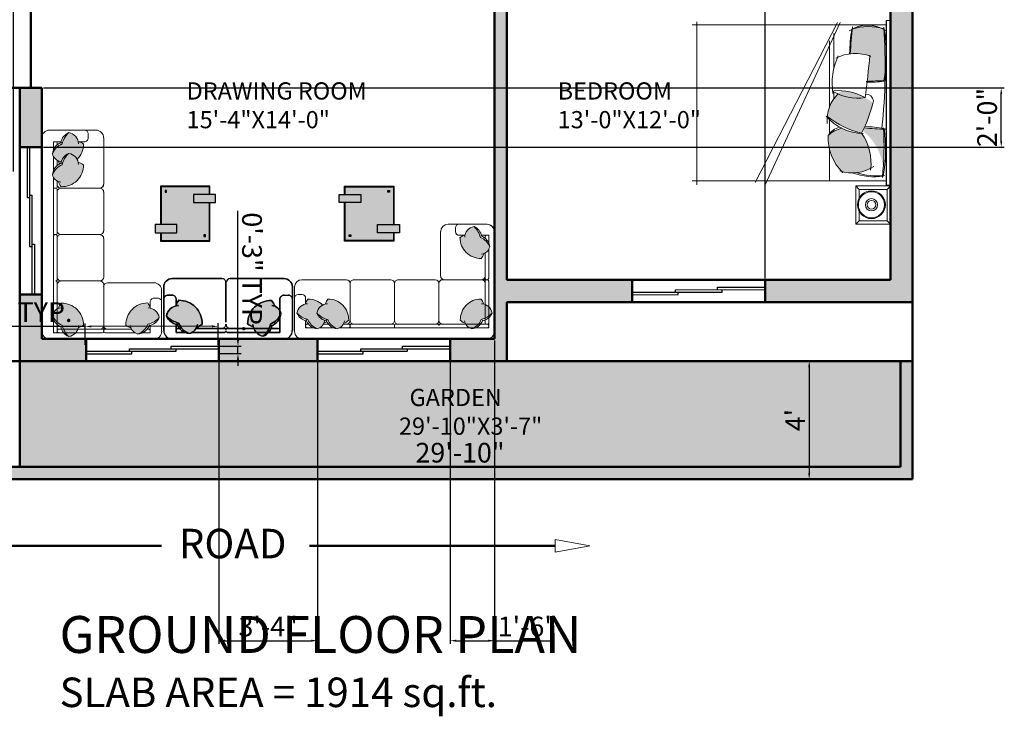
# Model space of a CAD drawing. Units: inches. Extents: x 1913 to 5309, y 1003 to 1733.
# Tile 14 of 23: x 4152 to 4552, y 1003 to 1286. Entities that reach past the tile are written whole.
import ezdxf

# ---------------------------------------------------------------- set-up
doc = ezdxf.new("R2010")
doc.units = ezdxf.units.IN
for name, color, linetype, lineweight in [('0.10', 252, 'Continuous', 9), ('0.15', 34, 'Continuous', 15), ('A-ANNO-DIMS', 2, 'Continuous', 18), ('A-ANNO-SYMB', 1, 'Continuous', 18), ('A-ANNO-TEXT', 7, 'Continuous', 18), ('A-AREA-IDEN', 3, 'Continuous', 18), ('A-DOOR', 4, 'Continuous', 25), ('A-FLOR-PATT', 252, 'Continuous', 13), ('A-FURN', 8, 'Continuous', 18), ('A-FURN-PATT', 8, 'Continuous', 13), ('A-GLAZ', 5, 'Continuous', 25), ('A-WALL', 7, 'Continuous', 50)]:
    doc.layers.add(name, color=color, linetype=linetype, lineweight=lineweight)
doc.layers.add('MOBIL', color=7, linetype='Continuous')
doc.styles.get("Standard").update_dxf_attribs({"font": 'arial.ttf'})
doc.dimstyles.new('ISO-25', dxfattribs={"dimtxt": 8, "dimasz": 2.5, "dimexe": 1.25, "dimexo": 0.625, "dimtad": 1, "dimdec": 1, "dimlunit": 3, "dimtxsty": 'Standard', "dimcen": 2.5, "dimclrd": 256, "dimclrt": 1, "dimadec": 0, "dimazin": 0, "dimtfac": 1, "dimtdec": 1, "dimtmove": 0, "dimatfit": 3, "dimfxl": 1, "dimarcsym": 0})

# ---------------------------------------------------------------- blocks, each defined once
blk = doc.blocks.new('Mesa de centro Cantria feeling')
at = {"layer": 'MOBIL', "ltscale": 0.2}
h = blk.add_hatch(color=256, dxfattribs=at)
h.set_gradient(color1=(74, 55, 38), color2=(104, 77, 54), one_color=1, tint=0.31, name='CYLINDER')
h.paths.add_polyline_path([(-0.85, -0.3), (-0.7, -0.3), (-0.7, 0.1), (-0.85, 0.1)])
h = blk.add_hatch(color=256, dxfattribs=at)
h.set_gradient(color1=(221, 221, 223), one_color=1, tint=1)
h.paths.add_polyline_path([(-0.15, -0.6), (-0.15, -0.89), (-0.01, -0.89), (-0.01, -0.01), (-0.7, -0.01), (-0.7, -0.3), (-0.85, -0.3), (-0.85, -0.01), (-0.99, -0.01), (-0.99, -0.89), (-0.3, -0.89), (-0.3, -0.6)])
h.paths.add_polyline_path([(-0.112, -0.112), (-0.112, -0.082), (-0.082, -0.082), (-0.082, -0.112)], flags=16)
h.paths.add_polyline_path([(-0.888, -0.788), (-0.888, -0.818), (-0.918, -0.818), (-0.918, -0.788)], flags=16)
h = blk.add_hatch(color=256, dxfattribs=at)
h.set_gradient(color1=(74, 55, 38), color2=(104, 77, 54), one_color=1, tint=0.31, name='CYLINDER')
h.paths.add_polyline_path([(-0.15, -0.6), (-0.3, -0.6), (-0.3, -1), (-0.15, -1)])
for points in [[(-0.85, 0), (-1, 0), (-1, -0.9), (-0.3, -0.9)], [(-0.15, -0.9), (0, -0.9), (0, 0), (-0.7, 0)], [(-0.85, -0.01), (-0.99, -0.01), (-0.99, -0.89), (-0.3, -0.89)], [(-0.15, -0.89), (-0.01, -0.89), (-0.01, -0.01), (-0.7, -0.01)]]:
    blk.add_lwpolyline(points, dxfattribs=at)
for points in [[(-0.85, -0.3), (-0.7, -0.3), (-0.7, 0.1), (-0.85, 0.1)], [(-0.082, -0.082), (-0.112, -0.082), (-0.112, -0.112), (-0.082, -0.112)], [(-0.15, -0.6), (-0.3, -0.6), (-0.3, -1), (-0.15, -1)], [(-0.918, -0.818), (-0.888, -0.818), (-0.888, -0.788), (-0.918, -0.788)]]:
    blk.add_lwpolyline(points, close=True, dxfattribs=at)
blk = doc.blocks.new('camita')
at = {"layer": '0.10'}
for p, q in [((-0.85, -0.045), (0.85, -0.045)), ((-0.805, -0.045), (-0.805, -2.048)), ((0.805, -0.045), (0.805, -2.048)), ((-0.827, -0.521), (0.846, -1.293)), ((-0.827, -0.548), (0.824, -1.399)), ((-0.716, -0.585), (-0.355, -0.585)), ((-0.114, -0.585), (-0.049, -0.585)), ((-0.638, -0.63), (0.043, -0.63)), ((0.175, -0.63), (0.318, -0.63)), ((0.474, -0.63), (0.805, -0.63)), ((-0.835, -2), (0.846, -2))]:
    blk.add_line(p, q, dxfattribs=at)
blk.add_lwpolyline([(-0.85, -0.041), (0.85, -0.041), (0.85, 0), (-0.85, 0)], close=True, dxfattribs=at)
for centre, radius, start, end in [((-0.457, -0.236), 0.344, 147.51, 213.8336), ((-0.2, -0.227), 0.586, 163.9263, 197.1409), ((-0.364, -5.846), 5.791, 83.8073, 94.1211), ((-0.51, -1.723), 1.678, 80.1255, 98.6619), ((2.353, -0.053), 2.58, 180.1063, 184.3854), ((-1.544, -0.245), 1.333, 359.9394, 7.5533), ((1.581, -0.289), 1.335, 170.3802, 178.9914), ((-1.44, -0.061), 1.712, 352.9291, 0.3959), ((0.452, -3.067), 3, 83.9026, 93.6759), ((0.486, -1.629), 1.578, 80.1602, 98.06), ((0.029, -0.138), 0.726, 342.5841, 6.0048), ((0.133, -0.17), 0.631, 339.923, 8.7433), ((-0.054, -0.363), 0.454, 159.3026, 206.5026), ((-0.007, -0.258), 0.0828, 100.018, 179.736), ((-0.293, -1.438), 1.29, 61.9749, 77.8435), ((0.627, -0.752), 0.551, 82.9691, 124.6739), ((0.32, -0.394), 0.404, 341.4524, 33.4512), ((-1.33, -9.675), 9.499, 82.2708, 84.9399), ((0.458, -0.545), 0.584, 151.0456, 184.1497), ((-0.534, -0.339), 0.487, 327.2644, 9.0473), ((-0.199, -0.274), 0.516, 310.7395, 359.0576), ((-0.567, -0.087), 0.906, 321.6953, 346.4626), ((-1.867, -14.986), 14.632, 84.6597, 85.7516), ((-0.46, 1.486), 1.909, 260.953, 268.6517), ((0.571, -0.432), 0.315, 192.9388, 221.9636), ((0.361, -0.133), 0.51, 267.2589, 315.2997), ((-0.2, 0.064), 0.667, 244.7809, 279.0606), ((0.179, -0.272), 0.383, 224.5284, 275.2229), ((0.438, -0.483), 0.19, 193.6849, 236.7035)]:
    blk.add_arc(centre, radius, start, end, dxfattribs=at)
blk = doc.blocks.new('VELADOR')
at = {"layer": '0.15'}
for p, q in [((-0.248, 0), (-0.203, -0.045)), ((0.248, 0), (0.202, -0.045)), ((-0.203, -0.405), (-0.248, -0.45)), ((0.248, -0.45), (0.202, -0.405))]:
    blk.add_line(p, q, dxfattribs=at)
blk.add_lwpolyline([(-0.248, 0), (-0.248, -0.45), (0.248, -0.45), (0.248, 0)], close=True, dxfattribs=at)
blk.add_lwpolyline([(0.092, -0.405), (0.202, -0.405), (0.202, -0.045), (-0.203, -0.045), (-0.203, -0.405), (-0.082, -0.405)], dxfattribs=at)
for radius in [0.18, 0.169, 0.0788, 0.0563]:
    blk.add_circle((0.005, -0.247), radius, dxfattribs=at)
blk = doc.blocks.new('d2 s')
at = {"transparency": 33554687}
h = blk.add_hatch(color=256, dxfattribs=at)
h.dxf.hatch_style = 1
h.paths.add_polyline_path([(3953.01, 1202.6, 0.213835), (3948.73, 1198.21, 0.233217), (3951.28, 1195.23, 0.122039), (3952.62, 1192.95, 0.425972), (3962.37, 1202.51, 0.156703), (3960.25, 1203.55), (3960.12, 1203.55, 0.310469), (3955.94, 1207.57, 0.147724)])
h = blk.add_hatch(color=256, dxfattribs=at)
h.dxf.hatch_style = 1
h.paths.add_polyline_path([(3953.9, 1162.75, -0.084911), (3952.59, 1164.92, -0.046133), (3950.85, 1165.51), (3950.85, 1171.8, -0.039409), (3951.63, 1172.02, -0.165523), (3952.68, 1174.28, -0.42585), (3962.24, 1164.53, -0.121928), (3959.96, 1163.19, -0.027403), (3959.75, 1162.75)])
h.paths.add_polyline_path([(3949.17, 1166.48), (3949.17, 1170.75, -0.097704), (3950.85, 1171.8), (3950.85, 1165.51, -0.04873)])
h.paths.add_polyline_path([(3947.62, 1167.84, -0.16488), (3949.17, 1170.75), (3949.17, 1166.48, -0.051917)])
h.paths.add_polyline_path([(3956, 1161.07, -0.090388), (3953.9, 1162.75), (3959.75, 1162.75, -0.136035), (3958.07, 1161.07)])
blk.add_line((3946.53, 1205.25), (3946.53, 1159.36), dxfattribs=at)
for p, q in [((3949.84, 1161.07), (3950.18, 1161.07)), ((3964.47, 1159.37), (3964.46, 1157.65))]:
    blk.add_line(p, q)
for points in [[(3955.94, 1207.57, 0.147724), (3953.01, 1202.6, 0.213355), (3948.73, 1198.22, -0.213355), (3953.01, 1202.6, -0.147724), (3955.94, 1207.57, 0.249545), (3952.4, 1203.17, -0.249545), (3955.93, 1207.59, -0.356779), (3960.22, 1202.7, 0.356779), (3955.94, 1207.57)], [(3948.72, 1198.23, 0.306333), (3952.42, 1194.91, -0.306333), (3948.72, 1198.23, -0.306674), (3952.79, 1203.29, 0.306674), (3948.72, 1198.23)], [(3952.62, 1192.95, 0.425972), (3962.37, 1202.51, 0.165552), (3960.12, 1203.57, -0.165552), (3962.37, 1202.51, -0.425972), (3952.63, 1192.95, -0.121514), (3951.29, 1195.22, 0.121514), (3952.62, 1192.95)], [(3947.62, 1167.84, 0.147724), (3952.59, 1164.92, 0.213355), (3956.97, 1160.64, -0.213355), (3952.59, 1164.92, -0.147724), (3947.62, 1167.84, 0.249545), (3952.02, 1164.3, -0.249545), (3947.61, 1167.84, -0.356779), (3952.49, 1172.13, 0.356779), (3947.62, 1167.84)], [(3962.24, 1164.53, 0.425972), (3952.68, 1174.28, 0.165552), (3951.63, 1172.02, -0.165552), (3952.68, 1174.28, -0.425972), (3962.24, 1164.53, -0.121514), (3959.97, 1163.19, 0.121514), (3962.24, 1164.53)], [(3956.96, 1160.63, 0.306333), (3960.28, 1164.33, -0.306333), (3956.96, 1160.63, -0.306674), (3951.9, 1164.7, 0.306674), (3956.96, 1160.63)]]:
    blk.add_lwpolyline(points, format="xyb", dxfattribs=at)
for points in [[(3949.93, 1208.66), (3967.86, 1208.66)], [(3949.17, 1203.55), (3952.49, 1203.55), (3949.17, 1203.55), (3949.17, 1199.96)], [(3960.13, 1203.55), (3962.77, 1203.55)], [(3964.46, 1205.25), (3964.46, 1206.96)], [(3971.27, 1205.25), (3971.27, 1184.84)], [(3950.85, 1202.87), (3950.85, 1202.25)], [(3949.17, 1197.14), (3949.17, 1183.83)], [(3950.85, 1195.43), (3950.85, 1183.83)], [(3950.99, 1183.17), (3950.65, 1183.17)], [(3969.63, 1183.17), (3953.36, 1183.17)], [(3949.17, 1164.09), (3949.17, 1182.51)], [(3950.85, 1161.74), (3950.85, 1182.51)], [(3971.25, 1181.39), (3971.25, 1159.35)], [(3949.17, 1161.07), (3949.17, 1164.4), (3949.17, 1161.07), (3952.75, 1161.07)], [(3952.75, 1161.06), (3962.77, 1161.06)], [(3949.93, 1155.95), (3967.86, 1155.95)]]:
    blk.add_lwpolyline(points, close=True, dxfattribs=at)
for points in [[(3962.76, 1208.66, -0.414214), (3964.46, 1206.97, 0.414214)], [(3967.85, 1208.66, -0.414212), (3971.25, 1205.26, 0.414212)], [(3950.18, 1203.55, -0.414214), (3950.85, 1202.88, 0.414214)], [(3964.46, 1205.26, -0.414214), (3962.76, 1203.57, 0.414214)], [(3964.47, 1159.37, 0.414214), (3962.77, 1161.06, -0.414214)], [(3967.85, 1155.95, 0.414212), (3971.25, 1159.35, -0.414212)], [(3962.76, 1155.95, 0.414214), (3964.46, 1157.65, -0.414214)]]:
    blk.add_lwpolyline(points, format="xyb", close=True, dxfattribs=at)
for centre, radius, start, end in [((3949.93, 1205.26), 3.4, 90.0002, 179.9998), ((3949.93, 1205.26), 3.4, 90.0846, 180.0842), ((3949.85, 1183.85), 0.681, 179.1575, 269.1575), ((3949.85, 1182.49), 0.681, 90.8425, 180.8425), ((3950.18, 1183.84), 0.671, 270, 0), ((3950.18, 1183.84), 0.671, 270, 0), ((3950.18, 1182.5), 0.671, 360, 90), ((3950.18, 1182.5), 0.671, 360, 90), ((3952.51, 1184.83), 1.66, 179.4889, 271.234), ((3952.51, 1181.52), 1.66, 88.766, 180.5111), ((3969.59, 1184.83), 1.66, 268.766, 0.5111), ((3969.39, 1181.32), 1.86, 2.0577, 84.9818), ((3969.39, 1181.32), 1.86, 2.0577, 84.9818), ((3969.59, 1184.83), 1.66, 268.7816, 0.5111), ((3949.93, 1159.36), 3.4, 180.0002, 269.9998), ((3949.93, 1159.37), 3.4, 180.0846, 270.0842), ((3949.84, 1161.74), 0.671, 180, 270), ((3950.18, 1161.74), 0.671, 270, 0)]:
    blk.add_arc(centre, radius, start, end, dxfattribs=at)
blk = doc.blocks.new('SOFA 1')
at = {"transparency": 33554687}
h = blk.add_hatch(color=256, dxfattribs=at)
h.dxf.hatch_style = 1
h.paths.add_polyline_path([(3723.52, 1308.63, 0.147724), (3717.76, 1305.24, 0.310469), (3722.42, 1300.4), (3722.42, 1300.25, 0.156703), (3723.62, 1297.8, 0.425821), (3734.69, 1309.08, 0.121928), (3732.05, 1310.63, 0.233216), (3728.6, 1313.59, 0.213835)])
h = blk.add_hatch(color=256, dxfattribs=at)
h.dxf.hatch_style = 1
h.paths.add_polyline_path([(3769.65, 1307.6, 0.084911), (3767.15, 1309.12, 0.046133), (3766.46, 1311.13), (3759.18, 1311.13, 0.039409), (3758.92, 1310.24, 0.165523), (3756.31, 1309.02, 0.42585), (3767.59, 1297.95, 0.121928), (3769.15, 1300.58, 0.027403), (3769.65, 1300.83)])
h.paths.add_polyline_path([(3765.34, 1313.08), (3760.4, 1313.08, 0.097704), (3759.18, 1311.13), (3766.46, 1311.13, 0.04873)])
h.paths.add_polyline_path([(3763.76, 1314.88, 0.16488), (3760.4, 1313.08), (3765.34, 1313.08, 0.051917)])
h.paths.add_polyline_path([(3771.6, 1305.17, 0.090388), (3769.65, 1307.6), (3769.65, 1300.83, 0.136035), (3771.6, 1302.77)])
h = blk.add_hatch(color=256, dxfattribs=at)
h.dxf.hatch_style = 1
h.paths.add_polyline_path([(3769.16, 1235.96, 0.122267), (3767.6, 1238.61, 0.425972), (3756.32, 1227.54, 0.165563), (3758.93, 1226.32, 0.309481), (3763.76, 1221.69, 0.002677), (3763.83, 1221.72, 0.146094), (3767.16, 1227.43, 0.212433), (3772.1, 1232.48, 0.235342)])
h = blk.add_hatch(color=256, dxfattribs=at)
h.dxf.hatch_style = 1
h.paths.add_polyline_path([(3769.16, 1225.36, 0.122267), (3767.6, 1228.01, 0.425972), (3756.32, 1216.94, 0.165563), (3758.93, 1215.72, 0.309481), (3763.76, 1211.09, 0.002677), (3763.83, 1211.12, 0.146094), (3767.16, 1216.83, 0.212433), (3772.1, 1221.88, 0.235342)])
for p, q in [((3720.45, 1316.13), (3773.58, 1316.13)), ((3777.51, 1312.19), (3777.51, 1213.72))]:
    blk.add_line(p, q, dxfattribs=at)
for points in [[(3717.76, 1305.24, -0.147724), (3723.52, 1308.63, -0.213355), (3728.59, 1313.59, 0.213355), (3723.52, 1308.63, 0.147724), (3717.76, 1305.24, -0.249545), (3722.86, 1309.34, 0.249545), (3717.75, 1305.25, 0.356779), (3723.4, 1300.28, -0.356779), (3717.76, 1305.24)], [(3728.58, 1313.6, -0.306333), (3732.42, 1309.31, 0.306333), (3728.58, 1313.6, 0.306674), (3722.72, 1308.89, -0.306674), (3728.58, 1313.6)], [(3763.76, 1314.88, -0.147724), (3767.15, 1309.12, -0.213355), (3772.1, 1304.05, 0.213355), (3767.15, 1309.12, 0.147724), (3763.76, 1314.88, -0.249545), (3767.86, 1309.77, 0.249545), (3763.77, 1314.89, 0.356779), (3758.8, 1309.23, -0.356779), (3763.76, 1314.88)], [(3734.69, 1309.08, -0.425972), (3723.62, 1297.8, -0.165552), (3722.4, 1300.4, 0.165552), (3723.62, 1297.79, 0.425972), (3734.69, 1309.07, 0.121514), (3732.07, 1310.63, -0.121514), (3734.69, 1309.08)], [(3767.6, 1297.95, -0.425972), (3756.31, 1309.01, -0.165552), (3758.92, 1310.24, 0.165552), (3756.31, 1309.02, 0.425972), (3767.59, 1297.95, 0.121514), (3769.14, 1300.57, -0.121514), (3767.6, 1297.95)], [(3772.11, 1304.06, -0.306333), (3767.83, 1300.22, 0.306333), (3772.11, 1304.06, 0.306674), (3767.4, 1309.91, -0.306674), (3772.11, 1304.06)], [(3770.44, 1286.63, -0.414214), (3769.66, 1287.4, 0.414214), (3770.44, 1286.63, 0.414214), (3769.66, 1285.83, -0.414214), (3770.44, 1286.63)], [(3748.01, 1262.99, -0.414214), (3746.05, 1264.95, 0.414214), (3748.01, 1262.97, 0.414213), (3746.05, 1261.01, -0.414213), (3748.01, 1262.99)], [(3770.44, 1262.99, -0.414214), (3769.66, 1263.77, 0.414214), (3770.44, 1262.99, 0.414214), (3769.66, 1262.19, -0.414214), (3770.44, 1262.99)], [(3770.83, 1262.97, -0.414214), (3771.61, 1262.19, 0.414214), (3770.83, 1262.99, 0.414214), (3771.61, 1263.77, -0.414214), (3770.83, 1262.97)], [(3748.01, 1239.35, -0.414214), (3746.05, 1241.31, 0.414214), (3748.01, 1239.33, 0.414213), (3746.05, 1237.37, -0.414213), (3748.01, 1239.35)], [(3756.32, 1227.54, -0.425972), (3767.6, 1238.61, -0.121514), (3769.16, 1235.98, 0.121514), (3767.6, 1238.61, 0.425972), (3756.32, 1227.54, 0.165552), (3758.93, 1226.32, -0.165552), (3756.32, 1227.54)], [(3767.7, 1239.33, -0.414214), (3769.66, 1237.37, 0.414214), (3767.7, 1239.35, 0.414214), (3769.66, 1241.31, -0.414214), (3767.7, 1239.33)], [(3770.44, 1239.35, -0.414214), (3769.66, 1240.13, 0.414214), (3770.44, 1239.33, 0.414214), (3769.66, 1238.55, -0.414214), (3770.44, 1239.35)], [(3770.83, 1239.33, -0.414214), (3771.61, 1238.55, 0.414214), (3770.83, 1239.35, 0.414214), (3771.61, 1240.13, -0.414214), (3770.83, 1239.33)], [(3772.1, 1232.5, -0.306674), (3767.41, 1226.64, 0.306674), (3772.1, 1232.5, 0.306333), (3767.84, 1236.34, -0.306333), (3772.1, 1232.5)], [(3763.78, 1221.67, 0.249545), (3767.87, 1226.78, -0.249545), (3763.76, 1221.69, -0.356779), (3758.81, 1227.32, 0.356779), (3763.77, 1221.68, 0.147724), (3767.16, 1227.43, 0.213355), (3772.11, 1232.51, -0.213355), (3767.16, 1227.43, -0.147724), (3763.78, 1221.67)], [(3756.32, 1216.94, -0.200233), (3759.49, 1224.76, 0.200233), (3756.32, 1216.94, 0.165552), (3758.93, 1215.72, -0.165552), (3756.32, 1216.94)], [(3772.1, 1221.9, -0.306674), (3767.41, 1216.04, 0.306674), (3772.1, 1221.9, -0.213355), (3767.16, 1216.83, -0.147724), (3763.77, 1211.08, 0.147724), (3767.15, 1216.83, 0.213355), (3772.1, 1221.9)], [(3763.76, 1211.09, -0.356779), (3758.81, 1216.72, 0.356779), (3763.76, 1211.09, 0.249545), (3767.87, 1216.18, -0.249545), (3763.76, 1211.09)]]:
    blk.add_lwpolyline(points, format="xyb", dxfattribs=at)
for points in [[(3716.51, 1312.2), (3716.51, 1291.44)], [(3722.42, 1313.08), (3722.42, 1309.23), (3722.42, 1313.08), (3726.57, 1313.08)], [(3723.21, 1311.13), (3723.93, 1311.13)], [(3729.85, 1313.08), (3745.25, 1313.08)], [(3731.82, 1311.13), (3745.25, 1311.13)], [(3746.01, 1312.3), (3746.01, 1288.55)], [(3746.01, 1310.97), (3746.01, 1311.36)], [(3746.01, 1288.54), (3746.01, 1308.23)], [(3768.11, 1313.08), (3746.78, 1313.08)], [(3768.87, 1311.13), (3746.78, 1311.13)], [(3771.6, 1313.08), (3767.75, 1313.08), (3771.6, 1313.08), (3771.6, 1308.93)], [(3769.66, 1287.39), (3769.65, 1312.3)], [(3769.65, 1309.43), (3769.65, 1308.71)], [(3771.6, 1313.08), (3771.61, 1233.74)], [(3722.42, 1300.39), (3722.42, 1297.33)], [(3720.45, 1295.38), (3718.48, 1295.38)], [(3720.45, 1287.5), (3744.09, 1287.5)], [(3746.02, 1284.63), (3746.02, 1264.94)], [(3747.99, 1286.6), (3767.69, 1286.6)], [(3769.66, 1263.75), (3769.66, 1285.81)], [(3769.66, 1277.18), (3769.66, 1263.75)], [(3746.02, 1260.99), (3746.02, 1241.3)], [(3747.99, 1262.97), (3767.69, 1262.97)], [(3769.66, 1240.12), (3769.66, 1262.18)], [(3770.43, 1262.97), (3770.82, 1262.97)], [(3747.99, 1239.33), (3767.69, 1239.33)], [(3769.66, 1235.71), (3769.66, 1238.54)], [(3770.43, 1239.33), (3770.82, 1239.33)], [(3746.02, 1237.36), (3746.02, 1213.74)], [(3771.61, 1223.14), (3771.61, 1230.47)], [(3769.66, 1225.11), (3769.66, 1227.82)], [(3767.76, 1215.72), (3771.61, 1215.72), (3771.61, 1219.84), (3771.61, 1215.72)], [(3753.91, 1211.77), (3753.91, 1213.74)], [(3755.86, 1215.72), (3758.92, 1215.72)], [(3769.66, 1216.5), (3769.66, 1217.22)], [(3749.97, 1209.8), (3773.58, 1209.8)]]:
    blk.add_lwpolyline(points, close=True, dxfattribs=at)
for points in [[(3722.42, 1311.91, 0.414214), (3723.2, 1311.13, -0.414214)], [(3770.43, 1313.08, 0.414214), (3769.65, 1312.3, -0.414214)], [(3771.6, 1312.3, 0.414214), (3770.82, 1313.08, -0.414214)], [(3716.51, 1297.34, 0.414214), (3718.47, 1295.38, -0.414214)], [(3720.44, 1295.38, 0.414214), (3722.4, 1297.34, -0.414214)], [(3716.51, 1291.45, 0.414212), (3720.44, 1287.52, -0.414212)], [(3746.03, 1288.56, 0.414214), (3747.99, 1286.6, 0.414213), (3746.03, 1284.64, -0.414213), (3747.99, 1286.6, -0.414214)], [(3769.66, 1284.64, 0.414214), (3767.7, 1286.6, 0.414214), (3769.66, 1288.56, -0.414214), (3767.7, 1286.6, -0.414214)], [(3769.66, 1261.01, 0.414214), (3767.7, 1262.97, 0.414214), (3769.66, 1264.93, -0.414214), (3767.7, 1262.97, -0.414214)], [(3772.13, 1221.9, 0.306333), (3767.84, 1225.74, -0.306333)], [(3769.16, 1225.36, 0.071861), (3768.39, 1227.01, -0.071861)], [(3746.05, 1213.76, 0.414212), (3749.98, 1209.82, -0.414212)], [(3755.87, 1215.72, 0.414214), (3753.91, 1213.76, -0.414214)], [(3769.66, 1216.52, 0.414214), (3770.44, 1215.74, -0.414214)], [(3770.83, 1215.74, 0.414214), (3771.61, 1216.52, -0.414214)], [(3755.87, 1209.8, -0.414214), (3753.91, 1211.76, 0.414214)]]:
    blk.add_lwpolyline(points, format="xyb", close=True, dxfattribs=at)
for centre, radius, start, end in [((3720.44, 1312.2), 3.93, 90.0002, 179.9998), ((3720.44, 1312.19), 3.94, 89.9158, 179.9154), ((3773.58, 1312.2), 3.93, 0.0002, 89.9998), ((3773.57, 1312.19), 3.94, 359.9158, 89.9154), ((3744.09, 1309.21), 1.92, 358.766, 90.5111), ((3745.22, 1312.29), 0.789, 0.8425, 90.8425), ((3745.24, 1311.91), 0.777, 270, 0), ((3745.24, 1311.91), 0.777, 270, 0), ((3746.8, 1312.29), 0.789, 89.1575, 179.1575), ((3746.79, 1311.91), 0.777, 180, 270), ((3746.79, 1311.91), 0.777, 180, 270), ((3747.93, 1309.21), 1.92, 89.4889, 181.234), ((3768.87, 1312.3), 0.777, 360, 90), ((3768.87, 1311.91), 0.777, 270, 0), ((3744.08, 1289.48), 1.96, 270, 360), ((3744.08, 1289.48), 1.96, 270, 360), ((3773.58, 1213.73), 3.93, 270.0002, 359.9998), ((3773.59, 1213.73), 3.93, 269.9156, 359.9152)]:
    blk.add_arc(centre, radius, start, end, dxfattribs=at)
blk = doc.blocks.new('*D18')
at = {"layer": 'A-ANNO-DIMS', "color": 0, "lineweight": -2, "transparency": 16777216}
for p, q in [((4473.78, 1146.96), (4474.41, 1146.96)), ((4473.16, 1144.46), (4473.16, 1101.46)), ((4473.78, 1098.96), (4474.41, 1098.96))]:
    blk.add_line(p, q, dxfattribs=at)
at = {"layer": 'A-ANNO-DIMS', "color": 0, "transparency": 16777216}
for points in [[(4472.74, 1144.46), (4473.57, 1144.46), (4473.16, 1146.96)], [(4472.74, 1101.46), (4473.57, 1101.46), (4473.16, 1098.96)]]:
    blk.add_solid(points, dxfattribs=at)
at = {"layer": 'Defpoints', "color": 0, "transparency": 16777216}
for p in [(4473.16, 1146.96), (4473.16, 1098.96), (4473.16, 1098.96)]:
    blk.add_point(p, dxfattribs=at)
at = {"layer": 'A-ANNO-DIMS', "color": 0, "transparency": 16777216, "insert": (4468.53, 1122.96), "char_height": 8, "attachment_point": 5, "rotation": 90}
blk.add_mtext("4'", dxfattribs=at)
blk = doc.blocks.new('*D19')
at = {"layer": 'A-ANNO-DIMS', "color": 0, "lineweight": -2, "transparency": 16777216}
for p, q in [((4152.21, 1104.59), (4152.21, 1105.21)), ((4510.21, 1104.59), (4510.21, 1105.21)), ((4507.71, 1103.96), (4154.71, 1103.96))]:
    blk.add_line(p, q, dxfattribs=at)
at = {"layer": 'A-ANNO-DIMS', "color": 0, "transparency": 16777216}
for points in [[(4154.71, 1104.38), (4154.71, 1103.55), (4152.21, 1103.96)], [(4507.71, 1104.38), (4507.71, 1103.55), (4510.21, 1103.96)]]:
    blk.add_solid(points, dxfattribs=at)
at = {"layer": 'Defpoints', "color": 0, "transparency": 16777216}
for p in [(4152.21, 1103.96), (4152.21, 1103.96), (4510.21, 1103.96)]:
    blk.add_point(p, dxfattribs=at)
at = {"layer": 'A-ANNO-DIMS', "color": 0, "transparency": 16777216, "insert": (4331.21, 1108.67), "char_height": 8, "attachment_point": 5}
blk.add_mtext('29\'-10"', dxfattribs=at)
blk = doc.blocks.new('WIN-54')
for p, q in [((0, 54), (0, 35)), ((1, 54), (1, 17)), ((0, 35), (1, 35)), ((1, 36), (2, 36)), ((2, 36), (2, 0)), ((1, 17), (2, 17)), ((2, 19), (3, 19)), ((3, 19), (3, 0))]:
    blk.add_line(p, q)
blk = doc.blocks.new('WIN-60')
for p, q in [((0, 60), (0, 39.5)), ((1, 60), (1, 19.5)), ((1, 40.5), (2, 40.5)), ((2, 40.5), (2, 0)), ((0, 39.5), (1, 39.5)), ((2, 20.5), (3, 20.5)), ((3, 20.5), (3, 0)), ((1, 19.5), (2, 19.5))]:
    blk.add_line(p, q)
blk = doc.blocks.new('*D57')
at = {"layer": 'A-ANNO-DIMS', "lineweight": -2, "transparency": 16777216}
for p, q in [((4178.83, 1161.04), (4073.85, 1160.96)), ((4230.33, 1161.08), (4181.33, 1161.05))]:
    blk.add_line(p, q, dxfattribs=at)
at = {"layer": 'A-ANNO-DIMS', "color": 0, "lineweight": -2, "transparency": 16777216}
for p, q in [((4178.84, 1153.57), (4178.83, 1162.29)), ((4232.84, 1153.61), (4232.83, 1162.33))]:
    blk.add_line(p, q, dxfattribs=at)
at = {"layer": 'A-ANNO-DIMS', "transparency": 16777216}
for points in [[(4181.33, 1161.46), (4181.33, 1160.63), (4178.83, 1161.04)], [(4230.33, 1161.5), (4230.33, 1160.67), (4232.83, 1161.08)]]:
    blk.add_solid(points, dxfattribs=at)
at = {"layer": 'Defpoints', "color": 0, "transparency": 16777216}
for p in [(4178.83, 1161.04), (4178.84, 1152.94), (4232.84, 1152.98)]:
    blk.add_point(p, dxfattribs=at)
at = {"layer": 'A-ANNO-DIMS', "color": 1, "transparency": 16777216, "insert": (4125.09, 1165.77), "char_height": 8, "attachment_point": 5, "rotation": 0.0441}
blk.add_mtext('WINDOW 4\'-6" TYP.', dxfattribs=at)
blk = doc.blocks.new('*D58')
at = {"layer": 'A-ANNO-DIMS', "lineweight": -2, "transparency": 16777216}
for p, q in [((4240.94, 1155.49), (4240.9, 1208)), ((4240.94, 1149.99), (4240.94, 1152.99)), ((4240.94, 1147.49), (4240.94, 1144.99))]:
    blk.add_line(p, q, dxfattribs=at)
at = {"layer": 'A-ANNO-DIMS', "color": 0, "lineweight": -2, "transparency": 16777216}
for p, q in [((4233.46, 1152.99), (4242.19, 1152.99)), ((4233.47, 1149.99), (4242.19, 1149.99))]:
    blk.add_line(p, q, dxfattribs=at)
at = {"layer": 'A-ANNO-DIMS', "transparency": 16777216}
for points in [[(4241.35, 1155.49), (4240.52, 1155.49), (4240.94, 1152.99)], [(4241.36, 1147.49), (4240.53, 1147.49), (4240.94, 1149.99)]]:
    blk.add_solid(points, dxfattribs=at)
at = {"layer": 'Defpoints', "color": 0, "transparency": 16777216}
for p in [(4232.84, 1152.98), (4240.94, 1152.99), (4232.84, 1149.98)]:
    blk.add_point(p, dxfattribs=at)
at = {"layer": 'A-ANNO-DIMS', "color": 1, "transparency": 16777216, "insert": (4245.63, 1183), "char_height": 8, "attachment_point": 5, "rotation": 270.0441}
blk.add_mtext('0\'-3" TYP.', dxfattribs=at)
blk = doc.blocks.new('*D59')
at = {"layer": 'A-ANNO-DIMS', "color": 0, "lineweight": -2, "transparency": 16777216}
for p, q in [((4152.59, 1352.96), (4148.36, 1352.96)), ((4152.59, 1328.96), (4148.36, 1328.96))]:
    blk.add_line(p, q, dxfattribs=at)
at = {"layer": 'A-ANNO-DIMS', "lineweight": -2, "transparency": 16777216}
for p, q in [((4149.61, 1350.46), (4149.61, 1331.46)), ((4149.61, 1328.96), (4149.61, 1223.98))]:
    blk.add_line(p, q, dxfattribs=at)
at = {"layer": 'A-ANNO-DIMS', "transparency": 16777216}
for points in [[(4149.2, 1350.46), (4150.03, 1350.46), (4149.61, 1352.96)], [(4149.2, 1331.46), (4150.03, 1331.46), (4149.61, 1328.96)]]:
    blk.add_solid(points, dxfattribs=at)
at = {"layer": 'Defpoints', "color": 0, "transparency": 16777216}
for p in [(4153.21, 1352.96), (4149.61, 1328.96), (4153.21, 1328.96)]:
    blk.add_point(p, dxfattribs=at)
at = {"layer": 'A-ANNO-DIMS', "color": 1, "transparency": 16777216, "insert": (4144.85, 1275.22), "char_height": 8, "attachment_point": 5, "rotation": 90}
blk.add_mtext('WINDOW 2\'-0" TYP.', dxfattribs=at)
blk = doc.blocks.new('*D111')
at = {"layer": 'A-ANNO-DIMS', "color": 0, "lineweight": -2, "transparency": 16777216}
for p, q in [((4327.21, 1155.34), (4327.21, 1032.04)), ((4345.21, 1155.34), (4345.21, 1032.04))]:
    blk.add_line(p, q, dxfattribs=at)
at = {"layer": 'A-ANNO-DIMS', "lineweight": -2, "transparency": 16777216}
for p, q in [((4329.71, 1033.29), (4342.71, 1033.29)), ((4345.21, 1033.29), (4369.48, 1033.29))]:
    blk.add_line(p, q, dxfattribs=at)
at = {"layer": 'A-ANNO-DIMS', "transparency": 16777216}
for points in [[(4329.71, 1033.7), (4329.71, 1032.87), (4327.21, 1033.29)], [(4342.71, 1033.7), (4342.71, 1032.87), (4345.21, 1033.29)]]:
    blk.add_solid(points, dxfattribs=at)
at = {"layer": 'Defpoints', "color": 0, "transparency": 16777216}
for p in [(4327.21, 1155.96), (4345.21, 1155.96), (4345.21, 1033.29)]:
    blk.add_point(p, dxfattribs=at)
at = {"layer": 'A-ANNO-DIMS', "color": 1, "transparency": 16777216, "insert": (4358.6, 1038), "char_height": 8, "attachment_point": 5}
blk.add_mtext('1\'-6"', dxfattribs=at)
blk = doc.blocks.new('*D112')
at = {"layer": 'A-ANNO-DIMS', "color": 0, "lineweight": -2, "transparency": 16777216}
for p, q in [((4233.21, 1146.34), (4233.21, 1032.04)), ((4273.21, 1146.34), (4273.21, 1032.04))]:
    blk.add_line(p, q, dxfattribs=at)
at = {"layer": 'A-ANNO-DIMS', "lineweight": -2, "transparency": 16777216}
blk.add_line((4235.71, 1033.29), (4270.71, 1033.29), dxfattribs=at)
at = {"layer": 'A-ANNO-DIMS', "transparency": 16777216}
for points in [[(4235.71, 1033.7), (4235.71, 1032.87), (4233.21, 1033.29)], [(4270.71, 1033.7), (4270.71, 1032.87), (4273.21, 1033.29)]]:
    blk.add_solid(points, dxfattribs=at)
at = {"layer": 'Defpoints', "color": 0, "transparency": 16777216}
for p in [(4233.21, 1146.96), (4273.21, 1146.96), (4273.21, 1033.29)]:
    blk.add_point(p, dxfattribs=at)
at = {"layer": 'A-ANNO-DIMS', "color": 1, "transparency": 16777216, "insert": (4253.21, 1038), "char_height": 8, "attachment_point": 5}
blk.add_mtext('3\'-4"', dxfattribs=at)
blk = doc.blocks.new('*D113')
at = {"layer": 'A-ANNO-DIMS', "color": 0, "lineweight": -2, "transparency": 16777216}
for p, q in [((4455.21, 1180.59), (4455.21, 1724.21)), ((4506.21, 1180.59), (4506.21, 1724.21))]:
    blk.add_line(p, q, dxfattribs=at)
at = {"layer": 'A-ANNO-DIMS', "lineweight": -2, "transparency": 16777216}
blk.add_line((4457.71, 1722.96), (4503.71, 1722.96), dxfattribs=at)
at = {"layer": 'A-ANNO-DIMS', "transparency": 16777216}
for points in [[(4457.71, 1723.38), (4457.71, 1722.55), (4455.21, 1722.96)], [(4503.71, 1723.38), (4503.71, 1722.55), (4506.21, 1722.96)]]:
    blk.add_solid(points, dxfattribs=at)
at = {"layer": 'Defpoints', "color": 0, "transparency": 16777216}
for p in [(4506.21, 1722.96), (4455.21, 1179.96), (4506.21, 1179.96)]:
    blk.add_point(p, dxfattribs=at)
at = {"layer": 'A-ANNO-DIMS', "color": 1, "transparency": 16777216, "insert": (4480.71, 1727.68), "char_height": 8, "attachment_point": 5}
blk.add_mtext('4\'-3"', dxfattribs=at)
blk = doc.blocks.new('*D114')
at = {"layer": 'A-ANNO-DIMS', "color": 0, "lineweight": -2, "transparency": 16777216}
for p, q in [((4161.84, 1257.96), (4552.46, 1257.96)), ((4161.84, 1233.96), (4552.46, 1233.96))]:
    blk.add_line(p, q, dxfattribs=at)
at = {"layer": 'A-ANNO-DIMS', "lineweight": -2, "transparency": 16777216}
blk.add_line((4551.21, 1236.46), (4551.21, 1255.46), dxfattribs=at)
at = {"layer": 'A-ANNO-DIMS', "transparency": 16777216}
for points in [[(4550.8, 1255.46), (4551.63, 1255.46), (4551.21, 1257.96)], [(4550.8, 1236.46), (4551.63, 1236.46), (4551.21, 1233.96)]]:
    blk.add_solid(points, dxfattribs=at)
at = {"layer": 'Defpoints', "color": 0, "transparency": 16777216}
for p in [(4161.21, 1257.96), (4551.21, 1257.96), (4161.21, 1233.96)]:
    blk.add_point(p, dxfattribs=at)
at = {"layer": 'A-ANNO-DIMS', "color": 1, "transparency": 16777216, "insert": (4546.5, 1245.96), "char_height": 8, "attachment_point": 5, "rotation": 90}
blk.add_mtext('2\'-0"', dxfattribs=at)

msp = doc.modelspace()

# ---------------------------------------------------------------- hatches: boundary and pattern name
at = {"layer": 'A-FLOR-PATT'}
h = msp.add_hatch(color=256, dxfattribs=at)
h.dxf.hatch_style = 1
h.paths.add_polyline_path([(3968.21, 1681.96), (3999.21, 1681.96), (3999.21, 1686.96), (3963.21, 1686.96), (3963.21, 1098.96), (4008.21, 1098.96), (4008.21, 1103.96), (3968.21, 1103.96)])
h.paths.add_polyline_path([(4515.21, 1146.96), (4510.21, 1146.96), (4510.21, 1103.96), (4128.21, 1103.96), (4128.21, 1098.96), (4515.21, 1098.96)])
h = msp.add_hatch(color=256, dxfattribs=at)
h.dxf.hatch_style = 1
h.paths.add_polyline_path([(4179.21, 1155.93), (4164.35, 1155.93, -0.035946), (4163.9, 1155.96), (4161.21, 1155.96), (4161.21, 1173.96), (4152.21, 1173.96), (4152.21, 1146.96), (4179.21, 1146.96)])
h.paths.add_polyline_path([(4273.21, 1155.96), (4266.93, 1155.96), (4233.21, 1155.96), (4233.21, 1146.96), (4273.21, 1146.96)])
h.paths.add_polyline_path([(4285.21, 1328.96), (4152.21, 1328.96), (4152.21, 1305.96), (4161.21, 1305.96), (4161.21, 1323.96), (4285.21, 1323.96)])
h.paths.add_polyline_path([(4161.21, 1257.96), (4152.21, 1257.96), (4152.21, 1233.96), (4161.21, 1233.96), (4161.21, 1237.71)])
h.paths.add_polyline_path([(4515.21, 1405.96), (4503.21, 1405.96), (4503.21, 1400.96), (4506.21, 1400.96), (4506.21, 1328.96), (4452.21, 1328.96), (4452.21, 1323.96), (4506.21, 1323.96), (4506.21, 1179.96), (4455.21, 1179.96), (4455.21, 1170.96), (4515.21, 1170.96)])
h.paths.add_polyline_path([(4157.21, 1686.96), (3999.21, 1686.96), (3999.21, 1625.96), (4008.21, 1625.96), (4008.21, 1677.96), (4152.21, 1677.96), (4152.21, 1554.96), (4157.21, 1554.96), (4157.21, 1599.96), (4225.21, 1599.96), (4225.21, 1608.96), (4157.21, 1608.96)])
h.paths.add_polyline_path([(4008.21, 1513.96), (4157.21, 1513.96), (4157.21, 1518.96), (4008.21, 1518.96), (4008.21, 1571.96), (3999.21, 1571.96), (3999.21, 1420.96), (4050.21, 1420.96), (4050.21, 1429.96), (4008.21, 1429.96)])
h.paths.add_polyline_path([(4157.21, 1477.96), (4152.21, 1477.96), (4152.21, 1429.96), (4110.21, 1429.96), (4110.21, 1420.96), (4157.21, 1420.96)], flags=17)
h.paths.add_polyline_path([(4350.21, 1608.96), (4345.21, 1608.96), (4321.21, 1608.96), (4321.21, 1599.96), (4350.21, 1599.96)])
h.paths.add_polyline_path([(4515.21, 1686.96), (4345.21, 1686.96), (4345.21, 1644.96), (4350.21, 1644.96), (4350.21, 1677.96), (4506.21, 1677.96), (4506.21, 1557.96), (4423.21, 1557.96), (4423.21, 1552.96), (4506.21, 1552.96), (4506.21, 1492.96), (4428.21, 1492.96), (4428.21, 1522.96), (4423.21, 1522.96), (4423.21, 1492.96), (4345.21, 1492.96), (4345.21, 1487.96), (4474.21, 1487.96), (4474.21, 1464.96), (4479.21, 1464.96), (4479.21, 1487.96), (4515.21, 1487.96)])
h.paths.add_polyline_path([(4479.21, 1428.96), (4474.21, 1428.96), (4474.21, 1405.96), (4345.21, 1405.96), (4345.21, 1358.96), (4350.21, 1358.96), (4350.21, 1400.96), (4417.21, 1400.96), (4417.21, 1394.96), (4422.21, 1394.96), (4422.21, 1400.96), (4479.21, 1400.96)])
h.paths.add_polyline_path([(4350.21, 1323.96), (4422.21, 1323.96), (4422.21, 1370.96), (4417.21, 1370.96), (4417.21, 1328.96), (4345.21, 1328.96), (4345.21, 1158.97, -0.414214), (4342.21, 1155.96), (4327.21, 1155.96), (4327.21, 1146.96), (4350.21, 1146.96), (4350.21, 1170.96), (4401.21, 1170.96), (4401.21, 1179.96), (4350.21, 1179.96)])
h.paths.add_polyline_path([(4157.21, 1356.96), (4152.21, 1356.96), (4152.21, 1352.96), (4157.21, 1352.96)])
h.paths.add_polyline_path([(4157.21, 1396.96), (4152.21, 1396.96), (4152.21, 1392.96), (4157.21, 1392.96)])
h = msp.add_hatch(color=256, dxfattribs=at)
h.dxf.hatch_style = 1
h.paths.add_polyline_path([(4510.21, 1103.96), (4510.21, 1146.96), (4152.21, 1146.96), (4152.21, 1103.96)])
h.paths.add_polyline_path([(4476.9, 1116.98), (4476.9, 1129.33), (4460.42, 1129.33), (4460.42, 1116.98)], flags=24)
h.paths.add_polyline_path([(4311.97, 1100.36), (4350.66, 1100.36), (4350.66, 1116.84), (4311.97, 1116.84)], flags=9)
h.paths.add_polyline_path([(4304.36, 1113.03), (4364.2, 1113.03), (4364.2, 1139.15), (4304.36, 1139.15)], flags=24)
at = {"layer": 'A-FURN-PATT'}
h = msp.add_hatch(color=256, dxfattribs=at)
h.dxf.hatch_style = 1
h.paths.add_polyline_path([(4489.79, 1271.86, -0.113891), (4497.78, 1270.99, -0.006967), (4496.71, 1260.63, -0.016701), (4503.49, 1260.9, 0.079172), (4503.73, 1281.69, 0.257422), (4490.64, 1282, -0.004417)])
h.paths.add_polyline_path([(4503.21, 1225.3, 0.033818), (4503.33, 1241.25, -0.041028), (4492.33, 1242.24, -0.246183)])
h = msp.add_hatch(color=256, dxfattribs=at)
h.dxf.hatch_style = 1
h.paths.add_polyline_path([(4494.45, 1239.63, 0.064806), (4499.06, 1251.91, 0.152135), (4486.31, 1256.86, 0.205841), (4480.51, 1246.46, 0.110131)])
h.paths.add_polyline_path([(4494.54, 1239.49, -0.104045), (4486.44, 1241.56, 0.127326), (4480.93, 1238.7, 0.202559), (4486.32, 1224.04, 0.194952), (4498.21, 1225.32, 0.173835)])

# ---------------------------------------------------------------- linework, layer by layer
at = {"layer": 'A-ANNO-SYMB'}
msp.add_lwpolyline([(4384.04, 1071.84), (4369.88, 1074.39), (4369.88, 1069.29)], close=True, dxfattribs=at)
at = {"layer": 'A-WALL'}
for p, q in [((4515.21, 1405.96), (4515.21, 1098.96)), ((4345.21, 1328.96), (4345.21, 1155.96)), ((4350.21, 1323.96), (4350.21, 1179.96)), ((4506.21, 1323.96), (4506.21, 1179.96)), ((4156.71, 1305.96), (4156.71, 1257.96)), ((4134.21, 1257.96), (4161.21, 1257.96)), ((4152.21, 1257.96), (4152.21, 1103.96)), ((4161.21, 1257.96), (4161.21, 1155.96)), ((4152.21, 1233.96), (4161.21, 1233.96)), ((4350.21, 1179.96), (4506.21, 1179.96)), ((4401.21, 1179.96), (4401.21, 1170.96)), ((4455.21, 1179.96), (4455.21, 1170.96)), ((4152.21, 1173.96), (4161.21, 1173.96)), ((4350.21, 1170.96), (4515.21, 1170.96)), ((4350.21, 1170.96), (4350.21, 1146.96)), ((4161.21, 1155.96), (4345.21, 1155.96)), ((4179.21, 1155.96), (4179.21, 1146.96)), ((4233.21, 1155.96), (4233.21, 1146.96)), ((4273.21, 1155.96), (4273.21, 1146.96)), ((4327.21, 1155.96), (4327.21, 1146.96)), ((4152.21, 1146.96), (3999.21, 1146.96)), ((4152.21, 1146.96), (4515.21, 1146.96)), ((4510.21, 1146.96), (4510.21, 1103.96)), ((4128.21, 1103.96), (4510.21, 1103.96)), ((4515.21, 1098.96), (4128.21, 1098.96)), ((4110.03, 1071.84), (4209.85, 1071.84)), ((4369.88, 1071.84), (4270.06, 1071.84))]:
    msp.add_line(p, q, dxfattribs=at)

# ---------------------------------------------------------------- block references
at = {"layer": 'A-DOOR', "xscale": 0.9914887765283156, "yscale": 0.9914887765283156, "zscale": 0.9914887765283156, "rotation": 90}
msp.add_blockref('d2 s', (5409.17, -2756.97), dxfattribs=at)
at = {"layer": 'A-FURN'}
for name, p, xscale, yscale, zscale, rotation in [('camita', (4506.21, 1251.96), 39.375, 39.375, 39.375, 270), ('SOFA 1', (7177.67, 2206.9), 0.7985303345031592, 0.7985303345031592, 0.7985303345031592, 180), ('Mesa de centro Cantria feeling', (4229.54, 1195.75), 22.3138190187957, 22.3138190187957, 22.3138190187957, 270), ('Mesa de centro Cantria feeling', (4284.26, 1195.75), -22.3138190187957, 22.3138190187957, 22.3138190187957, 90), ('VELADOR', (4506.21, 1210.35), -31.41542173157097, 31.41542173157097, 31.41542173157097, 269.9999999999999), ('SOFA 1', (3339.16, 4043.51), 0.7644053585719659, 0.7644053585719659, 0.7644053585719659, 270)]:
    msp.add_blockref(name, p, dxfattribs=dict(at, xscale=xscale, yscale=yscale, zscale=zscale, rotation=rotation))
at = {"layer": 'A-GLAZ'}
msp.add_blockref('WIN-60', (4155.21, 1173.96), dxfattribs=at)
for p, rotation in [((4454.84, 1173.98), 90.04407578688497), ((4232.84, 1149.98), 90.04407578688544), ((4326.84, 1149.98), 90.04407578688522)]:
    msp.add_blockref('WIN-54', p, dxfattribs=dict(at, rotation=rotation))

# ---------------------------------------------------------------- texts
at = {"layer": 'A-ANNO-TEXT', "attachment_point": 1}
for s, width, insert, char_height in [('  ROAD', 86.9528, (4209.58, 1078.77), 12), ('GROUND FLOOR PLAN\\P{\\H0.8x;SLAB AREA = 1914 sq.ft.}', 253.2094, (4168.42, 1043.3), 15)]:
    msp.add_mtext_dynamic_manual_height_columns(s, width=width, gutter_width=12.5, heights=[0], dxfattribs=dict(at, insert=insert, char_height=char_height))
at = {"layer": 'A-AREA-IDEN', "char_height": 7, "attachment_point": 1}
for s, insert in [('DRAWING ROOM 15\'-4"X14\'-0"', (4220.05, 1260.26)), ('BEDROOM\\P13\'-0"X12\'-0"', (4370.89, 1260.26)), ('  GARDEN\\P29\'-10"X3\'-7"', (4306.39, 1135.66))]:
    msp.add_mtext_dynamic_manual_height_columns(s, width=86.9528, gutter_width=12.5, heights=[0], dxfattribs=dict(at, insert=insert))

# ---------------------------------------------------------------- dimensions: what is measured, and where the dimension line sits
at = {"layer": 'A-ANNO-DIMS'}
for base, p1, p2, override, picture, middle in [((4506.21, 1722.96), (4455.21, 1179.96), (4506.21, 1179.96), {"dimdec": 1, "dimlfac": 1, "dimrnd": 0, "dimzin": 1, "dimdsep": 46, "dimlunit": 4, "dimfrac": 2}, '*D113', (4480.71, 1727.68)), ((4345.21, 1033.29), (4327.21, 1155.96), (4345.21, 1155.96), {"dimdec": 1, "dimlfac": 1, "dimrnd": 0, "dimzin": 1, "dimdsep": 46, "dimlunit": 4, "dimfrac": 2}, '*D111', (4358.6, 1038)), ((4273.21, 1033.29), (4233.21, 1146.96), (4273.21, 1146.96), {"dimdec": 1, "dimlfac": 1, "dimrnd": 0, "dimzin": 1, "dimdsep": 46, "dimlunit": 4, "dimfrac": 2}, '*D112', (4253.21, 1038)), ((4152.21, 1103.96), (4510.21, 1103.96), (4152.21, 1103.96), {"dimclrd": 0, "dimclre": 0, "dimclrt": 0}, '*D19', (4331.21, 1108.67))]:
    dim = msp.add_linear_dim(base=base, p1=p1, p2=p2, dimstyle='ISO-25', override=override, dxfattribs=at)
    dim.commit()
    dim.dimension.update_dxf_attribs({"geometry": picture, "text_midpoint": middle})
for base, p1, p2, angle, text, picture, middle in [((4149.61, 1328.96), (4153.21, 1352.96), (4153.21, 1328.96), 270, 'WINDOW <> TYP.', '*D59', (4144.85, 1275.22)), ((4240.94, 1152.99), (4232.84, 1149.98), (4232.84, 1152.98), 90.0441, '<> TYP.', '*D58', (4245.63, 1183)), ((4178.83, 1161.04), (4232.84, 1152.98), (4178.84, 1152.94), 180.0441, 'WINDOW <> TYP.', '*D57', (4125.09, 1165.77))]:
    dim = msp.add_linear_dim(base=base, p1=p1, p2=p2, angle=angle, text=text, dimstyle='ISO-25', override={"dimdec": 1, "dimrnd": 0, "dimzin": 1, "dimlunit": 4, "dimfrac": 2}, dxfattribs=at)
    dim.commit()
    dim.dimension.update_dxf_attribs({"geometry": picture, "text_midpoint": middle})
for base, p1, p2, override, picture, middle in [((4551.21, 1257.96), (4161.21, 1233.96), (4161.21, 1257.96), {"dimdec": 1, "dimlfac": 1, "dimrnd": 0, "dimzin": 1, "dimdsep": 46, "dimlunit": 4, "dimfrac": 2}, '*D114', (4546.5, 1245.96)), ((4473.16, 1098.96), (4473.16, 1146.96), (4473.16, 1098.96), {"dimclrd": 0, "dimclre": 0, "dimclrt": 0}, '*D18', (4468.53, 1122.96))]:
    dim = msp.add_linear_dim(base=base, p1=p1, p2=p2, angle=90, dimstyle='ISO-25', override=override, dxfattribs=at)
    dim.commit()
    dim.dimension.update_dxf_attribs({"geometry": picture, "text_midpoint": middle})

doc.saveas('drawing.dxf')
